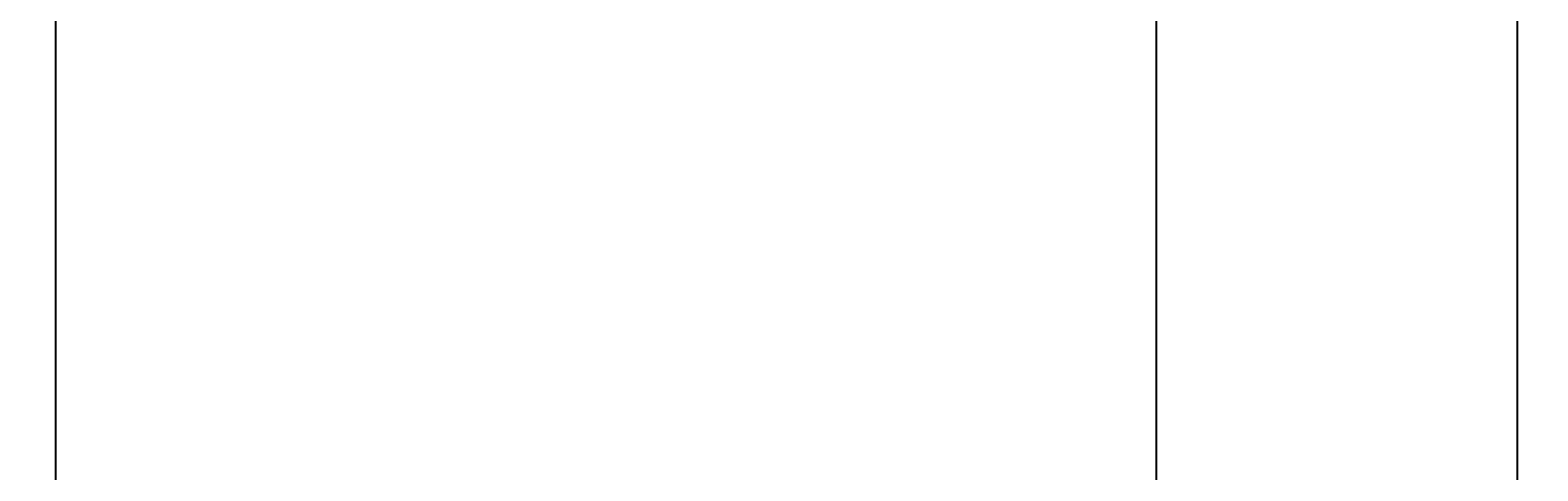
# Model space of a CAD drawing. Units: inches. Extents: x 35362 to 73946, y 43607 to 67532.
# Tile 57 of 134: x 50119 to 51337, y 46564 to 46919. Entities that reach past the tile are written whole.
import ezdxf

# ---------------------------------------------------------------- set-up
doc = ezdxf.new("R2010")
doc.units = ezdxf.units.IN
doc.header["$MEASUREMENT"] = 0
doc.layers.add('A-ANNO-DIMS', color=2, linetype='Continuous', lineweight=18)
doc.styles.get("Standard").update_dxf_attribs({"font": 'arial.ttf'})
doc.dimstyles.get("Standard").update_dxf_attribs({"dimtxt": 0.18, "dimasz": 0.18, "dimexe": 0.18, "dimexo": 0.0625, "dimgap": 0.09, "dimtad": 0, "dimtih": 1, "dimtoh": 1, "dimdec": 4, "dimzin": 0, "dimdsep": 46, "dimtxsty": 'Standard', "dimcen": 0.09, "dimadec": 0, "dimazin": 0, "dimtfac": 1, "dimtdec": 4, "dimtofl": 0, "dimtmove": 0, "dimatfit": 3, "dimfxl": 1, "dimtolj": 1, "dimtzin": 0, "dimarcsym": 0})

# ---------------------------------------------------------------- blocks, each defined once
blk = doc.blocks.new('*D5')
at = {"layer": 'A-ANNO-DIMS', "color": 0, "lineweight": -2, "transparency": 16777216}
for p, q in [((37121.9, 46919.3), (37121.9, 43606.7)), ((69871.5, 45449.8), (69871.5, 43606.7)), ((37122.1, 43606.9), (53496.3, 43606.9)), ((69871.3, 43606.9), (53497.2, 43606.9))]:
    blk.add_line(p, q, dxfattribs=at)
at = {"layer": 'A-ANNO-DIMS', "color": 0, "transparency": 16777216}
for points in [[(37122.1, 43606.9), (37122.1, 43606.8), (37121.9, 43606.9)], [(69871.3, 43606.9), (69871.3, 43606.8), (69871.5, 43606.9)]]:
    blk.add_solid(points, dxfattribs=at)
at = {"layer": 'Defpoints', "color": 0, "transparency": 16777216}
for p in [(37121.9, 46919.4), (69871.5, 45449.9), (69871.5, 43606.9)]:
    blk.add_point(p, dxfattribs=at)
at = {"layer": 'A-ANNO-DIMS', "color": 0, "transparency": 16777216, "insert": (53496.7, 43606.9), "char_height": 0.18, "attachment_point": 5}
blk.add_mtext('\\A1;32750', dxfattribs=at)
blk = doc.blocks.new('*D11')
at = {"layer": 'A-ANNO-DIMS', "color": 0, "lineweight": -2, "transparency": 16777216}
for p, q in [((47978.7, 56028.8), (47978.7, 43606.7)), ((53109.8, 56028.8), (53109.8, 43606.7)), ((47978.8, 43606.9), (50543.9, 43606.9)), ((53109.6, 43606.9), (50544.6, 43606.9))]:
    blk.add_line(p, q, dxfattribs=at)
at = {"layer": 'A-ANNO-DIMS', "color": 0, "transparency": 16777216}
for points in [[(47978.8, 43606.9), (47978.8, 43606.8), (47978.7, 43606.9)], [(53109.6, 43606.9), (53109.6, 43606.8), (53109.8, 43606.9)]]:
    blk.add_solid(points, dxfattribs=at)
at = {"layer": 'Defpoints', "color": 0, "transparency": 16777216}
for p in [(47978.7, 56028.8), (53109.8, 56028.8), (53109.8, 43606.9)]:
    blk.add_point(p, dxfattribs=at)
at = {"layer": 'A-ANNO-DIMS', "color": 0, "transparency": 16777216, "insert": (50544.2, 43606.9), "char_height": 0.18, "attachment_point": 5}
blk.add_mtext('\\A1;5131', dxfattribs=at)
blk = doc.blocks.new('*D13')
at = {"layer": 'A-ANNO-DIMS', "color": 0, "lineweight": -2, "transparency": 16777216}
for p, q in [((48373.5, 51694), (48373.5, 43606.7)), ((51029, 51694), (51029, 43606.7)), ((48373.7, 43606.9), (49700.8, 43606.9)), ((51028.9, 43606.9), (49701.7, 43606.9))]:
    blk.add_line(p, q, dxfattribs=at)
at = {"layer": 'A-ANNO-DIMS', "color": 0, "transparency": 16777216}
for points in [[(48373.7, 43606.9), (48373.7, 43606.8), (48373.5, 43606.9)], [(51028.9, 43606.9), (51028.9, 43606.8), (51029, 43606.9)]]:
    blk.add_solid(points, dxfattribs=at)
at = {"layer": 'Defpoints', "color": 0, "transparency": 16777216}
for p in [(48373.5, 51694.1), (51029, 51694.1), (51029, 43606.9)]:
    blk.add_point(p, dxfattribs=at)
at = {"layer": 'A-ANNO-DIMS', "color": 0, "transparency": 16777216, "insert": (49701.3, 43606.9), "char_height": 0.18, "attachment_point": 5}
blk.add_mtext('\\A1;2655.6', dxfattribs=at)
blk = doc.blocks.new('*D17')
at = {"layer": 'A-ANNO-DIMS', "color": 0, "lineweight": -2, "transparency": 16777216}
for p, q in [((49923.3, 61293.2), (49923.3, 43606.7)), ((51913.9, 61293.2), (51913.9, 43606.7)), ((49923.5, 43606.9), (50918.2, 43606.9)), ((51913.8, 43606.9), (50919.1, 43606.9))]:
    blk.add_line(p, q, dxfattribs=at)
at = {"layer": 'A-ANNO-DIMS', "color": 0, "transparency": 16777216}
for points in [[(49923.5, 43606.9), (49923.5, 43606.8), (49923.3, 43606.9)], [(51913.8, 43606.9), (51913.8, 43606.8), (51913.9, 43606.9)]]:
    blk.add_solid(points, dxfattribs=at)
at = {"layer": 'Defpoints', "color": 0, "transparency": 16777216}
for p in [(49923.3, 61293.3), (51913.9, 61293.3), (51913.9, 43606.9)]:
    blk.add_point(p, dxfattribs=at)
at = {"layer": 'A-ANNO-DIMS', "color": 0, "transparency": 16777216, "insert": (50918.6, 43606.9), "char_height": 0.18, "attachment_point": 5}
blk.add_mtext('\\A1;1990.6', dxfattribs=at)
blk = doc.blocks.new('*D67')
at = {"layer": 'A-ANNO-DIMS', "color": 0, "lineweight": -2, "transparency": 16777216}
for p, q in [((56873.5, 53351.5), (35361.8, 53351.5)), ((35361.9, 53351.3), (35361.9, 49400.9)), ((35361.9, 45450.1), (35361.9, 49400.5)), ((53793.6, 45449.9), (35361.8, 45449.9))]:
    blk.add_line(p, q, dxfattribs=at)
at = {"layer": 'A-ANNO-DIMS', "color": 0, "transparency": 16777216}
for points in [[(35361.9, 53351.3), (35362, 53351.3), (35361.9, 53351.5)], [(35361.9, 45450.1), (35362, 45450.1), (35361.9, 45449.9)]]:
    blk.add_solid(points, dxfattribs=at)
at = {"layer": 'Defpoints', "color": 0, "transparency": 16777216}
for p in [(35361.9, 53351.5), (56873.6, 53351.5), (53793.6, 45449.9)]:
    blk.add_point(p, dxfattribs=at)
at = {"layer": 'A-ANNO-DIMS', "color": 0, "transparency": 16777216, "insert": (35361.9, 49400.7), "char_height": 0.18, "attachment_point": 5}
blk.add_mtext('\\A1;7901.6', dxfattribs=at)
blk = doc.blocks.new('*D90')
at = {"layer": 'A-ANNO-DIMS', "color": 0, "lineweight": -2, "transparency": 16777216}
for p, q in [((53707.7, 47291.3), (35361.8, 47291.3)), ((35361.9, 47291.1), (35361.9, 46710.3)), ((35361.9, 46129.1), (35361.9, 46709.9)), ((53793.6, 46128.9), (35361.8, 46128.9))]:
    blk.add_line(p, q, dxfattribs=at)
at = {"layer": 'A-ANNO-DIMS', "color": 0, "transparency": 16777216}
for points in [[(35361.9, 47291.1), (35362, 47291.1), (35361.9, 47291.3)], [(35361.9, 46129.1), (35362, 46129.1), (35361.9, 46128.9)]]:
    blk.add_solid(points, dxfattribs=at)
at = {"layer": 'Defpoints', "color": 0, "transparency": 16777216}
for p in [(53707.8, 47291.3), (35361.9, 46128.9), (53793.6, 46128.9)]:
    blk.add_point(p, dxfattribs=at)
at = {"layer": 'A-ANNO-DIMS', "color": 0, "transparency": 16777216, "insert": (35361.9, 46710.1), "char_height": 0.18, "attachment_point": 5}
blk.add_mtext('\\A1;1162.4', dxfattribs=at)
blk = doc.blocks.new('*D107')
at = {"layer": 'A-ANNO-DIMS', "color": 0, "lineweight": -2, "transparency": 16777216}
for p, q in [((50139.6, 59850), (50139.6, 43606.7)), ((51320.8, 59850), (51320.8, 43606.7)), ((50139.7, 43606.9), (50729.7, 43606.9)), ((51320.6, 43606.9), (50730.6, 43606.9))]:
    blk.add_line(p, q, dxfattribs=at)
at = {"layer": 'A-ANNO-DIMS', "color": 0, "transparency": 16777216}
for points in [[(50139.7, 43606.9), (50139.7, 43606.8), (50139.6, 43606.9)], [(51320.6, 43606.9), (51320.6, 43606.8), (51320.8, 43606.9)]]:
    blk.add_solid(points, dxfattribs=at)
at = {"layer": 'Defpoints', "color": 0, "transparency": 16777216}
for p in [(50139.6, 59850.1), (51320.8, 59850.1), (51320.8, 43606.9)]:
    blk.add_point(p, dxfattribs=at)
at = {"layer": 'A-ANNO-DIMS', "color": 0, "transparency": 16777216, "insert": (50730.2, 43606.9), "char_height": 0.18, "attachment_point": 5}
blk.add_mtext('\\A1;1181.3', dxfattribs=at)

msp = doc.modelspace()

# ---------------------------------------------------------------- dimensions: what is measured, and where the dimension line sits
at = {"layer": 'A-ANNO-DIMS'}
for base, p1, p2, override, picture, middle in [((51913.931, 43606.859), (49923.307, 61293.286), (51913.931, 61293.286), {"dimdec": 1, "dimlfac": 1, "dimrnd": 0, "dimzin": 0, "dimdsep": 46, "dimlunit": 2}, '*D17', (50918.619, 43606.859)), ((51320.8133, 43606.859), (50139.5627, 59850.0769), (51320.8133, 59850.0769), {"dimdec": 1, "dimlfac": 1, "dimrnd": 0, "dimzin": 0, "dimdsep": 46, "dimlunit": 2}, '*D107', (50730.188, 43606.859)), ((53109.76, 43606.859), (47978.665, 56028.836), (53109.76, 56028.836), {"dimdec": 0, "dimlfac": 1, "dimrnd": 0, "dimzin": 0, "dimdsep": 46, "dimlunit": 2}, '*D11', (50544.212, 43606.859)), ((51029.043, 43606.859), (48373.492, 51694.087), (51029.043, 51694.087), {"dimdec": 1, "dimlfac": 1, "dimrnd": 0, "dimzin": 0, "dimdsep": 46, "dimlunit": 2}, '*D13', (49701.267, 43606.859)), ((69871.496, 43606.859), (37121.949, 46919.381), (69871.496, 45449.894), {"dimdec": 0, "dimlfac": 1, "dimrnd": 0, "dimzin": 0, "dimdsep": 46, "dimlunit": 2}, '*D5', (53496.723, 43606.859))]:
    dim = msp.add_linear_dim(base=base, p1=p1, p2=p2, dimstyle='Standard', override=override, dxfattribs=at)
    dim.commit()
    dim.dimension.update_dxf_attribs({"geometry": picture, "text_midpoint": middle})
for base, p1, p2, picture, middle in [((35361.949, 53351.529), (53793.638, 45449.894), (56873.602, 53351.529), '*D67', (35361.949, 49400.712)), ((35361.949, 46128.878), (53707.781, 47291.285), (53793.638, 46128.878), '*D90', (35361.949, 46710.081))]:
    dim = msp.add_linear_dim(base=base, p1=p1, p2=p2, angle=90, dimstyle='Standard', override={"dimdec": 1, "dimlfac": 1, "dimrnd": 0, "dimzin": 0, "dimdsep": 46, "dimlunit": 2}, dxfattribs=at)
    dim.commit()
    dim.dimension.update_dxf_attribs({"geometry": picture, "text_midpoint": middle})

doc.saveas('drawing.dxf')
